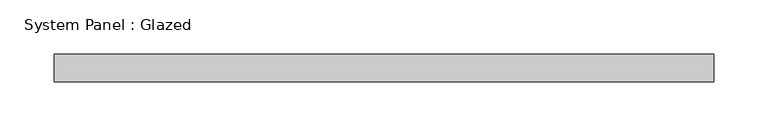
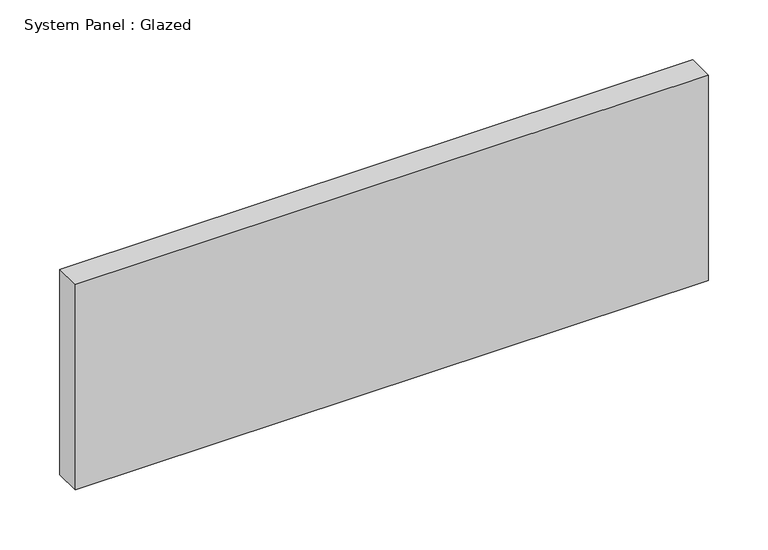
"""IFC4 building model written with IfcOpenShell, lengths in millimetres: plate geometry, System Panel : Glazed."""

from ifc_helpers import new_model, si_unit, origin, origin_with_axes, place, context, project, spatial, polyline, outline, extrude, source, transform, mapped, element, save


def system_panel_glazed_9fd37d83(model_context):
    return source(origin(), model_context, "Body", "SweptSolid", [
        extrude(outline(polyline([(304.8, 19.05), (-304.8, 19.05), (-304.8, 44.45), (304.8, 44.45), (304.8, 19.05)])), origin_with_axes(), (0.0, 0.0, 1.0), 209.55),
    ])


if __name__ == "__main__":
    model = new_model("IFC4")
    model_context = context("Model", 3, world=origin())
    ifc_project = project(units=[si_unit("LENGTHUNIT", "METRE", prefix="MILLI")], contexts=[model_context])
    site = spatial("IfcSite", under=ifc_project)
    building = spatial("IfcBuilding", under=site)
    placement = place(None, origin())
    system_panel_glazed_shape = system_panel_glazed_9fd37d83(model_context)
    element("IfcPlate", 1, ObjectType="System Panel : Glazed", at=placement, inside=building, context=model_context, shape_type="MappedRepresentation", body=[
        mapped(system_panel_glazed_shape, transform((0.0, 0.0, 0.0), x_axis=(1.0, 0.0, 0.0), y_axis=(0.0, 1.0, 0.0), z_axis=(0.0, 0.0, 1.0))),
    ])
    save(model, "model.ifc")

# Revit data of these elements
# Type "System Panel : Glazed"
#   Construction Type Id = "GSP4R"
#   Analytic Construction = "1/8 in Pilkington single glazing"
#   Visual Light Transmittance = 0.9
#   Solar Heat Gain Coefficient = 0.86
#   Heat Transfer Coefficient (U) = 1.18115 BTU/(h·ft²·°F)
#   Define Thermal Properties by = 1
# Element 1 (IfcPlate, "System Panel : Glazed")
#   Materials on its faces: "Glass"
# Materials
#   "Glass": class "Glass", colour RGB 0 128 192, transparency 0.75, Description = "Soda Lime Glass", Cost = 0
